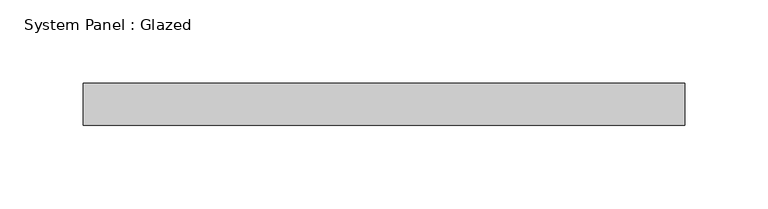
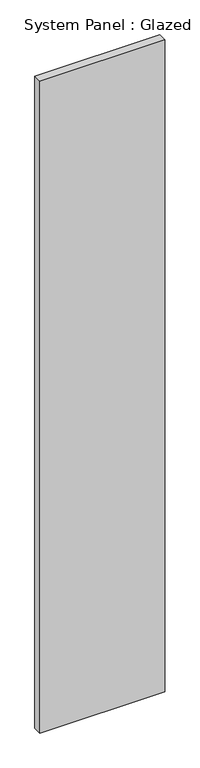
"""IFC4 building model written with IfcOpenShell, lengths in millimetres: plate geometry, System Panel : Glazed."""

from ifc_helpers import new_model, si_unit, origin, origin_with_axes, place, context, project, spatial, polyline, outline, extrude, source, transform, mapped, element, save


def system_panel_glazed_4f997f60(model_context):
    return source(origin(), model_context, "Body", "SweptSolid", [
        extrude(outline(polyline([(181.3019779, 19.05), (-181.3019779, 19.05), (-181.3019779, 44.45), (181.3019779, 44.45), (181.3019779, 19.05)])), origin_with_axes(), (0.0, 0.0, 1.0), 2003.0999183),
    ])


if __name__ == "__main__":
    model = new_model("IFC4")
    model_context = context("Model", 3, world=origin())
    ifc_project = project(units=[si_unit("LENGTHUNIT", "METRE", prefix="MILLI")], contexts=[model_context])
    site = spatial("IfcSite", under=ifc_project)
    building = spatial("IfcBuilding", under=site)
    placement = place(None, origin())
    system_panel_glazed_shape = system_panel_glazed_4f997f60(model_context)
    element("IfcPlate", 1, ObjectType="System Panel : Glazed", at=placement, inside=building, context=model_context, shape_type="MappedRepresentation", body=[
        mapped(system_panel_glazed_shape, transform((0.0, 0.0, 0.0), x_axis=(1.0, 0.0, 0.0), y_axis=(0.0, 1.0, 0.0), z_axis=(0.0, 0.0, 1.0))),
    ])
    save(model, "model.ifc")

# Revit data of these elements
# Type "System Panel : Glazed"
#   Construction Type Id = "GSP4R"
#   Analytic Construction = "1/8 in Pilkington single glazing"
#   Visual Light Transmittance = 0.9
#   Solar Heat Gain Coefficient = 0.86
#   Heat Transfer Coefficient (U) = 1.18115 BTU/(h·ft²·°F)
#   Define Thermal Properties by = 1
# Element 1 (IfcPlate, "System Panel : Glazed")
#   Materials on its faces: "Glass"
# Materials
#   "Glass": class "Glass", colour RGB 154 182 205, transparency 0.85, Description = "Soda Lime Glass", Cost = 0
